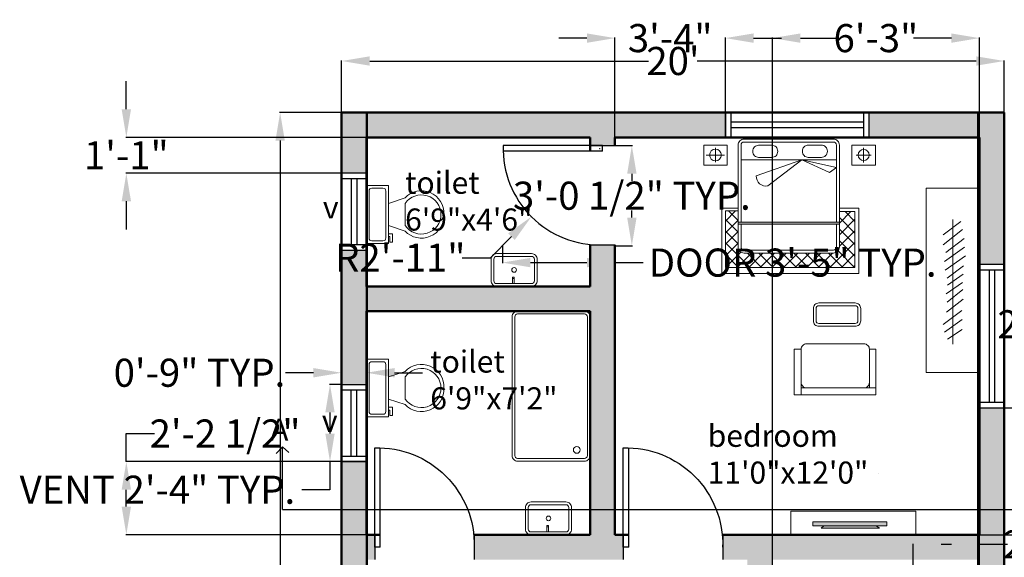
# Model space of a CAD drawing. Units: inches. Extents: x 4451 to 5261, y 886 to 1442.
# Tile 2 of 4: x 4451 to 4807, y 1247 to 1442. Entities that reach past the tile are written whole.
import ezdxf

# ---------------------------------------------------------------- set-up
doc = ezdxf.new("R2010")
doc.units = ezdxf.units.IN
doc.header["$MEASUREMENT"] = 0
for name, color, linetype, lineweight in [('A-ANNO-DIMS', 2, 'Continuous', 18), ('A-ANNO-SYMB', 3, 'Continuous', 25), ('A-ANNO-TEXT', 7, 'Continuous', 25), ('A-AREA-IDEN', 7, 'Continuous', 25), ('A-DOOR', 4, 'Continuous', 25), ('A-FLOR-FIXT', 9, 'Continuous', 20), ('A-FURN', 8, 'Continuous', 18), ('A-FURN-PATT', 8, 'Continuous', 13), ('A-GLAZ', 4, 'Continuous', 25), ('A-WALL', 7, 'Continuous', 50), ('A-WALL-PATT', 252, 'Continuous', 13)]:
    doc.layers.add(name, color=color, linetype=linetype, lineweight=lineweight)
doc.styles.get("Standard").update_dxf_attribs({"font": 'arial.ttf'})
doc.dimstyles.get("Standard").update_dxf_attribs({"dimtxt": 10.18, "dimasz": 10.18, "dimexe": 0.18, "dimexo": 0.0625, "dimgap": 0.09, "dimtad": 0, "dimtih": 1, "dimtoh": 1, "dimdec": 0, "dimzin": 0, "dimdsep": 46, "dimlunit": 3, "dimtxsty": 'Standard', "dimcen": 0.09, "dimadec": 0, "dimazin": 0, "dimtfac": 1, "dimtdec": 0, "dimtofl": 0, "dimtmove": 0, "dimatfit": 3, "dimfxl": 1, "dimtolj": 1, "dimtzin": 0, "dimarcsym": 0})
pattern_1 = [(45, (-374.59908, -99.02593), (-0.095474584, 0.095474584), []), (135, (-374.59908, -99.02593), (-0.2864237525, 0.095474584), [0.33755363, -0.202532178])]

# ---------------------------------------------------------------- blocks, each defined once
blk = doc.blocks.new('*U3')
for p, q in [((9.5, -6), (9.5, -2)), ((-10, -8.5), (-8, -8.5)), ((-10, -9.5), (-10, -8.5)), ((-7, -9.5), (-10, -9.5)), ((-8, -8.5), (-8, -8)), ((-7, -8), (-7, -9.5)), ((-4, -8), (-6, -14)), ((4, -8), (6, -14)), ((4, -14), (-4, -14))]:
    blk.add_line(p, q)
blk.add_lwpolyline([(10.5, -8), (10.5, 0), (-10.5, 0), (-10.5, -8)], close=True)
for points in [[(-9.5, -2), (-9.5, -6)], [(8.5, -1), (-8.5, -1)], [(-8.5, -7), (8.5, -7)]]:
    blk.add_lwpolyline(points)
for centre, radius, start, end in [((-8.625, -1.875), 0.8839, 81.8699, 188.1301), ((8.625, -1.875), 0.8839, 351.8699, 98.1301), ((-8.625, -6.125), 0.8839, 171.869898, 278.1301), ((8.625, -6.125), 0.8839, 261.8699, 8.1301), ((-0.4772, -19.9188), 8.0953, 133.01722, 273.38), ((0.0374, -19.8731), 7.127, 124.50543, 269.7), ((-0.0373, -19.8731), 7.127, 270.3, 55.4946), ((0.4773, -19.9188), 8.0953, 266.62, 46.9828)]:
    blk.add_arc(centre, radius, start, end)
blk = doc.blocks.new('*D11')
at = {"layer": 'A-ANNO-DIMS', "color": 0, "lineweight": -2, "transparency": 16777216}
for p, q in [((4567.09, 1408.31), (4567.09, 1427.09)), ((4577.27, 1426.91), (4678.28, 1426.91)), ((4796.91, 1426.91), (4695.91, 1426.91)), ((4807.09, 1408.31), (4807.09, 1427.09))]:
    blk.add_line(p, q, dxfattribs=at)
at = {"layer": 'A-ANNO-DIMS', "color": 0, "transparency": 16777216}
for points in [[(4577.27, 1428.6), (4577.27, 1425.21), (4567.09, 1426.91)], [(4796.91, 1428.6), (4796.91, 1425.21), (4807.09, 1426.91)]]:
    blk.add_solid(points, dxfattribs=at)
at = {"layer": 'Defpoints', "color": 0, "transparency": 16777216}
for p in [(4807.09, 1426.91), (4567.09, 1408.25), (4807.09, 1408.25)]:
    blk.add_point(p, dxfattribs=at)
at = {"layer": 'A-ANNO-DIMS', "color": 0, "transparency": 16777216, "insert": (4687.09, 1426.91), "char_height": 10.18, "attachment_point": 5}
blk.add_mtext("\\A1;20'", dxfattribs=at)
blk = doc.blocks.new('*D12')
at = {"layer": 'A-ANNO-DIMS', "color": 0, "lineweight": -2, "transparency": 16777216}
for p, q in [((4567.03, 1408.25), (4544.66, 1408.25)), ((4544.84, 1398.07), (4544.84, 1173.54)), ((4544.84, 938.43), (4544.84, 1162.96)), ((4567.03, 928.25), (4544.66, 928.25))]:
    blk.add_line(p, q, dxfattribs=at)
at = {"layer": 'A-ANNO-DIMS', "color": 0, "transparency": 16777216}
for points in [[(4543.14, 1398.07), (4546.53, 1398.07), (4544.84, 1408.25)], [(4543.14, 938.43), (4546.53, 938.43), (4544.84, 928.25)]]:
    blk.add_solid(points, dxfattribs=at)
at = {"layer": 'Defpoints', "color": 0, "transparency": 16777216}
for p in [(4567.09, 1408.25), (4544.84, 928.25), (4567.09, 928.25)]:
    blk.add_point(p, dxfattribs=at)
at = {"layer": 'A-ANNO-DIMS', "color": 0, "transparency": 16777216, "insert": (4544.84, 1168.25), "char_height": 10.18, "attachment_point": 5}
blk.add_mtext("\\A1;40'", dxfattribs=at)
blk = doc.blocks.new('DOOR-36-SWING')
for p, q in [((36.01, 36.01), (0.01, 36.01)), ((31.51, 36.01), (40.51, 36.01)), ((36.01, 34.01), (36.01, 36.01)), ((36.01, 34.01), (0.01, 34.01)), ((31.51, 0.01), (40.51, 0.01))]:
    blk.add_line(p, q)
blk.add_arc((35.01, 35.01), 35.01, 178.3634, 271.6366)
blk = doc.blocks.new('WIN-48-PLAN')
for p, q in [((0, 52), (9, 52)), ((0, 50), (9, 50)), ((3.5, 50), (3.5, 2)), ((5.5, 50), (5.5, 2)), ((0, 2), (9, 2)), ((0, 0), (9, 0))]:
    blk.add_line(p, q)
blk = doc.blocks.new('VENT-24-PLAN')
for p, q in [((9, 28), (0, 28)), ((9, 26), (0, 26)), ((3.5, 26), (3.5, 2)), ((5.5, 26), (5.5, 2)), ((9, 2), (0, 2)), ((9, 0), (0, 0))]:
    blk.add_line(p, q)
blk = doc.blocks.new('*D23')
at = {"layer": 'A-ANNO-DIMS', "color": 0, "lineweight": -2, "transparency": 16777216}
for p, q in [((4625.32, 1359.91), (4625.32, 1353.68)), ((4666.09, 1359.91), (4666.09, 1353.68)), ((4635.5, 1353.86), (4655.91, 1353.86)), ((4666.09, 1353.86), (4676.27, 1353.86))]:
    blk.add_line(p, q, dxfattribs=at)
at = {"layer": 'A-ANNO-DIMS', "color": 0, "transparency": 16777216}
for points in [[(4635.5, 1355.56), (4635.5, 1352.16), (4625.32, 1353.86)], [(4655.91, 1355.56), (4655.91, 1352.16), (4666.09, 1353.86)]]:
    blk.add_solid(points, dxfattribs=at)
at = {"layer": 'Defpoints', "color": 0, "transparency": 16777216}
for p in [(4625.32, 1359.98), (4666.09, 1359.98), (4666.09, 1353.86)]:
    blk.add_point(p, dxfattribs=at)
at = {"layer": 'A-ANNO-DIMS', "color": 0, "transparency": 16777216, "insert": (4730.44, 1353.86), "char_height": 10.18, "attachment_point": 5}
blk.add_mtext('\\A1;DOOR 3\'-5" TYP.', dxfattribs=at)
blk = doc.blocks.new('*D24')
at = {"layer": 'A-ANNO-DIMS', "color": 0, "lineweight": -2, "transparency": 16777216}
for p, q in [((4666.16, 1396.25), (4672.39, 1396.25)), ((4672.21, 1386.07), (4672.21, 1383.47)), ((4672.21, 1370.16), (4672.21, 1372.76)), ((4666.16, 1359.98), (4672.39, 1359.98))]:
    blk.add_line(p, q, dxfattribs=at)
at = {"layer": 'A-ANNO-DIMS', "color": 0, "transparency": 16777216}
for points in [[(4670.51, 1386.07), (4673.91, 1386.07), (4672.21, 1396.25)], [(4670.51, 1370.16), (4673.91, 1370.16), (4672.21, 1359.98)]]:
    blk.add_solid(points, dxfattribs=at)
at = {"layer": 'Defpoints', "color": 0, "transparency": 16777216}
for p in [(4666.09, 1396.25), (4672.21, 1396.25), (4666.09, 1359.98)]:
    blk.add_point(p, dxfattribs=at)
at = {"layer": 'A-ANNO-DIMS', "color": 0, "transparency": 16777216, "insert": (4672.21, 1378.11), "char_height": 10.18, "attachment_point": 5}
blk.add_mtext('\\A1;3\'-0 1/2" TYP.', dxfattribs=at)
blk = doc.blocks.new('*D25')
at = {"layer": 'A-ANNO-DIMS', "color": 0, "lineweight": -2, "transparency": 16777216}
for p, q in [((4567.03, 1309.75), (4562.71, 1309.75)), ((4562.89, 1299.57), (4562.89, 1291.93)), ((4567.03, 1281.75), (4562.71, 1281.75)), ((4562.89, 1281.75), (4562.89, 1271.57)), ((4562.89, 1271.57), (4552.71, 1271.57))]:
    blk.add_line(p, q, dxfattribs=at)
at = {"layer": 'A-ANNO-DIMS', "color": 0, "transparency": 16777216}
for points in [[(4561.2, 1299.57), (4564.59, 1299.57), (4562.89, 1309.75)], [(4561.2, 1291.93), (4564.59, 1291.93), (4562.89, 1281.75)]]:
    blk.add_solid(points, dxfattribs=at)
at = {"layer": 'Defpoints', "color": 0, "transparency": 16777216}
for p in [(4567.09, 1309.75), (4562.89, 1281.75), (4567.09, 1281.75)]:
    blk.add_point(p, dxfattribs=at)
at = {"layer": 'A-ANNO-DIMS', "color": 0, "transparency": 16777216, "insert": (4500.39, 1271.57), "char_height": 10.18, "attachment_point": 5}
blk.add_mtext('\\A1;VENT 2\'-4" TYP.', dxfattribs=at)
blk = doc.blocks.new('*D26')
at = {"layer": 'A-ANNO-DIMS', "color": 0, "lineweight": -2, "transparency": 16777216}
for p, q in [((4556.91, 1313.95), (4546.73, 1313.95)), ((4567.09, 1309.81), (4567.09, 1314.13)), ((4576.09, 1309.81), (4576.09, 1314.13)), ((4586.27, 1313.95), (4596.45, 1313.95))]:
    blk.add_line(p, q, dxfattribs=at)
at = {"layer": 'A-ANNO-DIMS', "color": 0, "transparency": 16777216}
for points in [[(4556.91, 1315.65), (4556.91, 1312.26), (4567.09, 1313.95)], [(4586.27, 1315.65), (4586.27, 1312.26), (4576.09, 1313.95)]]:
    blk.add_solid(points, dxfattribs=at)
at = {"layer": 'Defpoints', "color": 0, "transparency": 16777216}
for p in [(4567.09, 1313.95), (4567.09, 1309.75), (4576.09, 1309.75)]:
    blk.add_point(p, dxfattribs=at)
at = {"layer": 'A-ANNO-DIMS', "color": 0, "transparency": 16777216, "insert": (4515.62, 1313.95), "char_height": 10.18, "attachment_point": 5}
blk.add_mtext('\\A1;0\'-9" TYP.', dxfattribs=at)
blk = doc.blocks.new('*D41')
at = {"layer": 'A-ANNO-DIMS', "color": 0, "lineweight": -2, "transparency": 16777216}
for p, q in [((4723.09, 1102.31), (4723.09, 1435.38)), ((4733.27, 1435.2), (4746.94, 1435.2)), ((4787.91, 1435.2), (4774.24, 1435.2)), ((4798.09, 1102.31), (4798.09, 1435.38))]:
    blk.add_line(p, q, dxfattribs=at)
at = {"layer": 'A-ANNO-DIMS', "color": 0, "transparency": 16777216}
for points in [[(4733.27, 1436.9), (4733.27, 1433.51), (4723.09, 1435.2)], [(4787.91, 1436.9), (4787.91, 1433.51), (4798.09, 1435.2)]]:
    blk.add_solid(points, dxfattribs=at)
at = {"layer": 'Defpoints', "color": 0, "transparency": 16777216}
for p in [(4798.09, 1435.2), (4723.09, 1102.25), (4798.09, 1102.25)]:
    blk.add_point(p, dxfattribs=at)
at = {"layer": 'A-ANNO-DIMS', "color": 0, "transparency": 16777216, "insert": (4760.59, 1435.2), "char_height": 10.18, "attachment_point": 5}
blk.add_mtext('\\A1;6\'-3"', dxfattribs=at)
blk = doc.blocks.new('*D46')
at = {"layer": 'A-ANNO-DIMS', "color": 0, "lineweight": -2, "transparency": 16777216}
for p, q in [((4798.16, 1301.25), (4859.61, 1301.25)), ((4859.43, 1291.07), (4859.43, 1283.54)), ((4859.43, 1265.43), (4859.43, 1272.96)), ((4798.16, 1255.25), (4859.61, 1255.25))]:
    blk.add_line(p, q, dxfattribs=at)
at = {"layer": 'A-ANNO-DIMS', "color": 0, "transparency": 16777216}
for points in [[(4857.74, 1291.07), (4861.13, 1291.07), (4859.43, 1301.25)], [(4857.74, 1265.43), (4861.13, 1265.43), (4859.43, 1255.25)]]:
    blk.add_solid(points, dxfattribs=at)
at = {"layer": 'Defpoints', "color": 0, "transparency": 16777216}
for p in [(4798.09, 1301.25), (4859.43, 1301.25), (4798.09, 1255.25)]:
    blk.add_point(p, dxfattribs=at)
at = {"layer": 'A-ANNO-DIMS', "color": 0, "transparency": 16777216, "insert": (4859.43, 1278.25), "char_height": 10.18, "attachment_point": 5}
blk.add_mtext('\\A1;3\'-10"', dxfattribs=at)
blk = doc.blocks.new('*D47')
at = {"layer": 'A-ANNO-DIMS', "color": 0, "lineweight": -2, "transparency": 16777216}
for p, q in [((4655.91, 1435.2), (4645.73, 1435.2)), ((4666.09, 1399.31), (4666.09, 1435.38)), ((4706.09, 1399.31), (4706.09, 1435.38)), ((4716.27, 1435.2), (4726.45, 1435.2))]:
    blk.add_line(p, q, dxfattribs=at)
at = {"layer": 'A-ANNO-DIMS', "color": 0, "transparency": 16777216}
for points in [[(4655.91, 1436.9), (4655.91, 1433.51), (4666.09, 1435.2)], [(4716.27, 1436.9), (4716.27, 1433.51), (4706.09, 1435.2)]]:
    blk.add_solid(points, dxfattribs=at)
at = {"layer": 'Defpoints', "color": 0, "transparency": 16777216}
for p in [(4706.09, 1435.2), (4666.09, 1399.25), (4706.09, 1399.25)]:
    blk.add_point(p, dxfattribs=at)
at = {"layer": 'A-ANNO-DIMS', "color": 0, "transparency": 16777216, "insert": (4686.09, 1435.2), "char_height": 10.18, "attachment_point": 5}
blk.add_mtext('\\A1;3\'-4"', dxfattribs=at)
blk = doc.blocks.new('*D49')
at = {"layer": 'A-ANNO-DIMS', "color": 0, "lineweight": -2, "transparency": 16777216}
for p, q in [((4489.14, 1281.75), (4489.14, 1291.93)), ((4489.14, 1291.93), (4499.32, 1291.93)), ((4576.03, 1281.75), (4488.96, 1281.75)), ((4489.14, 1265.43), (4489.14, 1271.57)), ((4576.03, 1255.25), (4488.96, 1255.25))]:
    blk.add_line(p, q, dxfattribs=at)
at = {"layer": 'A-ANNO-DIMS', "color": 0, "transparency": 16777216}
for points in [[(4487.45, 1271.57), (4490.84, 1271.57), (4489.14, 1281.75)], [(4487.45, 1265.43), (4490.84, 1265.43), (4489.14, 1255.25)]]:
    blk.add_solid(points, dxfattribs=at)
at = {"layer": 'Defpoints', "color": 0, "transparency": 16777216}
for p in [(4489.14, 1281.75), (4576.09, 1281.75), (4576.09, 1255.25)]:
    blk.add_point(p, dxfattribs=at)
at = {"layer": 'A-ANNO-DIMS', "color": 0, "transparency": 16777216, "insert": (4524.89, 1291.93), "char_height": 10.18, "attachment_point": 5}
blk.add_mtext('\\A1;2\'-2 1/2"', dxfattribs=at)
blk = doc.blocks.new('*D50')
at = {"layer": 'A-ANNO-DIMS', "color": 0, "lineweight": -2, "transparency": 16777216}
for p, q in [((4489.14, 1409.43), (4489.14, 1419.61)), ((4576.03, 1399.25), (4488.96, 1399.25)), ((4576.03, 1386.25), (4488.96, 1386.25)), ((4489.14, 1376.07), (4489.14, 1365.89))]:
    blk.add_line(p, q, dxfattribs=at)
at = {"layer": 'A-ANNO-DIMS', "color": 0, "transparency": 16777216}
for points in [[(4487.45, 1409.43), (4490.84, 1409.43), (4489.14, 1399.25)], [(4487.45, 1376.07), (4490.84, 1376.07), (4489.14, 1386.25)]]:
    blk.add_solid(points, dxfattribs=at)
at = {"layer": 'Defpoints', "color": 0, "transparency": 16777216}
for p in [(4576.09, 1399.25), (4489.14, 1386.25), (4576.09, 1386.25)]:
    blk.add_point(p, dxfattribs=at)
at = {"layer": 'A-ANNO-DIMS', "color": 0, "transparency": 16777216, "insert": (4489.14, 1392.75), "char_height": 10.18, "attachment_point": 5}
blk.add_mtext('\\A1;1\'-1"', dxfattribs=at)
blk = doc.blocks.new('*D54')
at = {"layer": 'A-ANNO-DIMS', "color": 0, "lineweight": -2, "transparency": 16777216}
for p, q in [((4774.09, 1224.89), (4774.09, 1251.96)), ((4784.27, 1251.78), (4787.91, 1251.78)), ((4798.09, 1224.89), (4798.09, 1251.96)), ((4798.09, 1251.78), (4808.27, 1251.78))]:
    blk.add_line(p, q, dxfattribs=at)
at = {"layer": 'A-ANNO-DIMS', "color": 0, "transparency": 16777216}
for points in [[(4784.27, 1253.48), (4784.27, 1250.08), (4774.09, 1251.78)], [(4787.91, 1253.48), (4787.91, 1250.08), (4798.09, 1251.78)]]:
    blk.add_solid(points, dxfattribs=at)
at = {"layer": 'Defpoints', "color": 0, "transparency": 16777216}
for p in [(4798.09, 1251.78), (4774.09, 1224.83), (4798.09, 1224.83)]:
    blk.add_point(p, dxfattribs=at)
at = {"layer": 'A-ANNO-DIMS', "color": 0, "transparency": 16777216, "insert": (4821.98, 1251.78), "char_height": 10.18, "attachment_point": 5}
blk.add_mtext('\\A1;2\'-0"', dxfattribs=at)
blk = doc.blocks.new('*D61')
at = {"layer": 'A-ANNO-DIMS', "color": 0, "lineweight": -2, "transparency": 16777216}
for p, q in [((4860.41, 1349.3), (4835.61, 1349.3)), ((4835.79, 1339.12), (4835.79, 1336.87)), ((4835.79, 1323.9), (4835.79, 1326.16)), ((4880.22, 1313.72), (4835.61, 1313.72))]:
    blk.add_line(p, q, dxfattribs=at)
at = {"layer": 'A-ANNO-DIMS', "color": 0, "transparency": 16777216}
for points in [[(4834.09, 1339.12), (4837.48, 1339.12), (4835.79, 1349.3)], [(4834.09, 1323.9), (4837.48, 1323.9), (4835.79, 1313.72)]]:
    blk.add_solid(points, dxfattribs=at)
at = {"layer": 'Defpoints', "color": 0, "transparency": 16777216}
for p in [(4835.79, 1349.3), (4860.47, 1349.3), (4880.28, 1313.72)]:
    blk.add_point(p, dxfattribs=at)
at = {"layer": 'A-ANNO-DIMS', "color": 0, "transparency": 16777216, "insert": (4835.79, 1331.51), "char_height": 10.18, "attachment_point": 5}
blk.add_mtext('\\A1;2\'-11 1/2"', dxfattribs=at)
blk = doc.blocks.new('*D81')
at = {"layer": 'A-ANNO-DIMS', "color": 0, "lineweight": -2, "transparency": 16777216}
for p, q in [((4660.5, 1395.25), (4660.68, 1395.25)), ((4660.59, 1395.16), (4660.59, 1395.34)), ((4620.98, 1355.64), (4628.64, 1363.3)), ((4610.8, 1355.64), (4620.98, 1355.64))]:
    blk.add_line(p, q, dxfattribs=at)
at = {"layer": 'A-ANNO-DIMS', "color": 0, "transparency": 16777216}
blk.add_solid([(4627.44, 1364.49), (4629.84, 1362.1), (4635.83, 1370.49)], dxfattribs=at)
at = {"layer": 'Defpoints', "color": 0, "transparency": 16777216}
for p in [(4660.59, 1395.25), (4635.83, 1370.49)]:
    blk.add_point(p, dxfattribs=at)
at = {"layer": 'A-ANNO-DIMS', "color": 0, "transparency": 16777216, "insert": (4588.35, 1355.64), "char_height": 10.18, "attachment_point": 5}
blk.add_mtext('\\A1;R2\'-11"', dxfattribs=at)

msp = doc.modelspace()

# ---------------------------------------------------------------- hatches: boundary and pattern name
at = {"layer": 'A-FURN-PATT'}
h = msp.add_hatch(dxfattribs=at)
h.set_pattern_fill('ANSI37', color=256, scale=23.763776)
h.set_pattern_definition([(45, (-374.599, -99.026), (-2.1004409, 2.1004409), []), (135, (-374.599, -99.026), (-2.1004409, -2.1004409), [])])
h.paths.add_polyline_path([(4753, 1352.14), (4753, 1372.36), (4747.37, 1372.36), (4747.37, 1359.46, -0.414214), (4745.2, 1357.3), (4712.84, 1357.3, -0.414214), (4710.68, 1359.46), (4710.68, 1372.58), (4706.09, 1372.58), (4706.09, 1352.14)])
h = msp.add_hatch(dxfattribs=at)
h.set_pattern_fill('ANSI38', color=256, scale=1.080172)
h.set_pattern_definition(pattern_1)
h.paths.add_polyline_path([(4711.76, 1368.56), (4710.68, 1368.56), (4710.68, 1367.77), (4711.76, 1367.77)])
h.paths.add_polyline_path([(4747.37, 1368.56), (4746.29, 1368.56), (4746.29, 1367.77), (4747.37, 1367.77)])
h = msp.add_hatch(dxfattribs=at)
h.set_pattern_fill('ANSI38', color=256, scale=1.080172)
h.set_pattern_definition(pattern_1)
h.paths.add_polyline_path([(4746.29, 1368.56), (4711.76, 1368.56), (4711.76, 1367.77), (4746.29, 1367.77)])
h = msp.add_hatch(color=256, dxfattribs=at)
h.dxf.hatch_style = 1
h.paths.add_polyline_path([(4764.53, 1259.92), (4737.8, 1259.92), (4737.8, 1258.54), (4764.53, 1258.54)])
h.paths.add_polyline_path([(4760.66, 1258.54), (4741.71, 1258.54), (4740.83, 1257.67), (4761.95, 1257.67)])
at = {"layer": 'A-WALL-PATT'}
h = msp.add_hatch(color=256, dxfattribs=at)
h.dxf.hatch_style = 1
h.paths.add_polyline_path([(4706.09, 1408.25), (4567.09, 1408.25), (4567.09, 1386.25), (4576.09, 1386.25), (4576.09, 1399.25), (4657.09, 1399.25), (4657.09, 1396.25), (4661.59, 1396.25), (4666.09, 1396.25), (4666.09, 1399.25), (4706.09, 1399.25)])
h.paths.add_polyline_path([(4807.09, 1408.25), (4758.09, 1408.25), (4758.09, 1399.25), (4798.09, 1399.25), (4798.09, 1353.25), (4807.09, 1353.25)])
h.paths.add_polyline_path([(4807.09, 1301.25), (4798.09, 1301.25), (4798.09, 1292.89), (4798.09, 1255.25), (4705.09, 1255.25), (4705.09, 1252.75, -0.014283), (4705.09, 1250.75), (4705.09, 1246.25), (4714.09, 1246.25), (4714.09, 1243.25), (4723.09, 1243.25), (4723.09, 1246.25), (4798.09, 1246.25), (4798.09, 1200.25), (4807.09, 1200.25)])
h.paths.add_polyline_path([(4666.09, 1360.25), (4661.59, 1360.25, -0.014283), (4659.59, 1360.25), (4657.09, 1360.25), (4657.09, 1345.25), (4576.09, 1345.25), (4576.09, 1358.25), (4567.09, 1358.25), (4567.09, 1309.75), (4576.09, 1309.75), (4576.09, 1336.25), (4657.09, 1336.25), (4657.09, 1255.25), (4615.09, 1255.25), (4615.09, 1252.75, -0.014283), (4615.09, 1250.75), (4615.09, 1246.25), (4669.09, 1246.25), (4669.09, 1255.25), (4666.09, 1255.25)])
h.paths.add_polyline_path([(4576.09, 1281.75), (4567.09, 1281.75), (4567.09, 1211.26), (4576.09, 1211.26), (4576.09, 1246.25), (4579.09, 1246.25), (4579.09, 1255.25), (4576.09, 1255.25)])
h.paths.add_polyline_path([(4666.09, 1102.25), (4576.09, 1102.25), (4576.09, 1159.26), (4567.09, 1159.26), (4567.09, 928.25), (4596.54, 928.25), (4596.54, 937.25), (4576.09, 937.25), (4576.09, 1093.25), (4579.09, 1093.25), (4657.09, 1093.25), (4657.09, 982.46), (4666.09, 982.46), (4666.09, 1093.25)])
h.paths.add_polyline_path([(4723.09, 1207.25), (4720.59, 1207.25, -0.014283), (4718.59, 1207.25), (4714.09, 1207.25), (4714.09, 1102.25), (4711.09, 1102.25), (4711.09, 1097.75), (4711.09, 1093.25), (4734.59, 1093.25), (4734.59, 1102.25), (4723.09, 1102.25)])
h.paths.add_polyline_path([(4807.09, 1148.25), (4798.09, 1148.25), (4798.09, 1102.25), (4786.59, 1102.25), (4786.59, 1093.25), (4798.09, 1093.25), (4798.09, 1041.25), (4807.09, 1041.25)])
h.paths.add_polyline_path([(4694.85, 937.25), (4649.53, 937.25), (4648.54, 937.25), (4648.54, 928.25), (4649.53, 928.25), (4694.85, 928.25)])
h.paths.add_polyline_path([(4807.09, 989.25), (4798.09, 989.25), (4798.09, 937.25), (4798.09, 928.25), (4807.09, 928.25)])
h.paths.add_polyline_path([(4662.88, 1033.63), (4722.94, 1033.63), (4722.94, 1063.48), (4662.88, 1063.48)], flags=9)

# ---------------------------------------------------------------- linework, layer by layer
at = {"layer": 'A-ANNO-SYMB'}
for p, q in [((4545.71, 1287.14), (4543.39, 1284.64)), ((4545.71, 1264.36), (4545.71, 1287.14)), ((4545.71, 1287.14), (4547.97, 1285.05)), ((4545.71, 1264.36), (4671.09, 1264.36)), ((4671.09, 1264.36), (4828.9, 1264.36))]:
    msp.add_line(p, q, dxfattribs=at)
at = {"layer": 'A-FLOR-FIXT'}
for points in [[(4621.23, 1355.12, -0.414214), (4623.23, 1357.12), (4635.9, 1357.12, -0.414214), (4637.9, 1355.12), (4637.9, 1347.25, -0.414214), (4635.9, 1345.25), (4623.23, 1345.25, -0.414214), (4621.23, 1347.25)], [(4622.23, 1355.12, -0.414214), (4623.23, 1356.12), (4635.9, 1356.12, -0.414214), (4636.9, 1355.12), (4636.9, 1347.25, -0.414214), (4635.9, 1346.25), (4623.23, 1346.25, -0.414214), (4622.23, 1347.25)], [(4657.09, 1334.25, 0.414214), (4655.09, 1336.25), (4630.84, 1336.25, 0.414214), (4628.84, 1334.25), (4628.84, 1283.91, 0.414214), (4630.84, 1281.91), (4655.09, 1281.91, 0.414214), (4657.09, 1283.91)], [(4656.09, 1334.25, 0.414214), (4655.09, 1335.25), (4630.84, 1335.25, 0.414214), (4629.84, 1334.25), (4629.84, 1283.91, 0.414214), (4630.84, 1282.91), (4655.09, 1282.91, 0.414214), (4656.09, 1283.91)], [(4633.69, 1265.12, -0.414214), (4635.69, 1267.12), (4648.35, 1267.12, -0.414214), (4650.35, 1265.12), (4650.35, 1257.25, -0.414214), (4648.35, 1255.25), (4635.69, 1255.25, -0.414214), (4633.69, 1257.25)], [(4634.69, 1265.12, -0.414214), (4635.69, 1266.12), (4648.35, 1266.12, -0.414214), (4649.35, 1265.12), (4649.35, 1257.25, -0.414214), (4648.35, 1256.25), (4635.69, 1256.25, -0.414214), (4634.69, 1257.25)]]:
    msp.add_lwpolyline(points, format="xyb", close=True, dxfattribs=at)
for points in [[(4629.57, 1346.25), (4629.57, 1346.25), (4629.01, 1346.25), (4629.01, 1346.25), (4629.01, 1348.57), (4629.01, 1348.57), (4629.57, 1348.57), (4629.57, 1348.57)], [(4629.01, 1348.57), (4629.01, 1348.57), (4629.57, 1348.57), (4629.57, 1348.57), (4629.57, 1348.09), (4629.57, 1348.09), (4629.01, 1348.09), (4629.01, 1348.09)], [(4642.02, 1256.25), (4642.02, 1256.25), (4641.46, 1256.25), (4641.46, 1256.25), (4641.46, 1258.57), (4641.46, 1258.57), (4642.02, 1258.57), (4642.02, 1258.57)], [(4641.46, 1258.57), (4641.46, 1258.57), (4642.02, 1258.57), (4642.02, 1258.57), (4642.02, 1258.09), (4642.02, 1258.09), (4641.46, 1258.09), (4641.46, 1258.09)]]:
    msp.add_lwpolyline(points, close=True, dxfattribs=at)
for centre, radius in [((4629.57, 1351.19), 0.842), ((4652.26, 1286), 1.24), ((4642.02, 1261.19), 0.842)]:
    msp.add_circle(centre, radius, dxfattribs=at)
at = {"layer": 'A-FURN'}
for p, q in [((4702.49, 1395.43), (4702.49, 1390.2)), ((4756.16, 1395.39), (4756.16, 1390.13)), ((4699.09, 1392.84), (4705.75, 1392.84)), ((4733.74, 1391.08), (4717.27, 1385.27)), ((4721.43, 1381.68), (4733.74, 1391.08)), ((4746.29, 1388.3), (4733.74, 1391.08)), ((4733.74, 1391.08), (4743.74, 1386.47)), ((4753.49, 1392.76), (4758.93, 1392.76)), ((4743.74, 1386.47), (4746.29, 1388.3)), ((4710.68, 1373.61), (4704.82, 1373.61)), ((4704.82, 1373.61), (4704.82, 1349.9)), ((4710.68, 1373.61), (4710.68, 1373.61)), ((4754.45, 1373.61), (4747.37, 1373.61)), ((4754.45, 1349.9), (4754.45, 1373.61)), ((4710.68, 1372.58), (4706.09, 1372.58)), ((4706.09, 1372.58), (4706.09, 1352.14)), ((4747.37, 1372.36), (4753, 1372.36)), ((4753, 1372.36), (4753, 1352.14)), ((4788.46, 1369.51), (4788.46, 1324.32)), ((4710.68, 1368.56), (4747.37, 1368.56)), ((4710.68, 1367.77), (4747.37, 1367.77)), ((4785.01, 1363.88), (4791.36, 1368.8)), ((4785.01, 1360.32), (4791.9, 1365.88)), ((4785.9, 1357.5), (4792.6, 1362.65)), ((4785.44, 1354.28), (4792.67, 1359.5)), ((4785.67, 1351.13), (4793.06, 1356.27)), ((4706.09, 1352.14), (4753, 1352.14)), ((4786.44, 1348.28), (4792.36, 1352.66)), ((4704.82, 1349.9), (4754.45, 1349.9)), ((4786.55, 1345.65), (4792.21, 1349.66)), ((4785.99, 1342.51), (4791.96, 1346.62)), ((4786.43, 1339.53), (4792.11, 1344.12)), ((4786.14, 1335.91), (4792.16, 1340.6)), ((4784.95, 1331.43), (4791.71, 1336.55)), ((4785.48, 1328.62), (4791.87, 1333.26)), ((4786.47, 1326.14), (4791.82, 1329.65)), ((4760.51, 1308.43), (4760.51, 1305.99)), ((4741.71, 1258.54), (4739.83, 1258.54)), ((4741.71, 1258.54), (4740.83, 1257.67)), ((4740.83, 1257.67), (4761.95, 1257.67)), ((4761.95, 1257.67), (4760.66, 1258.54))]:
    msp.add_line(p, q, dxfattribs=at)
for points in [[(4710.68, 1396.46, -0.414214), (4712.84, 1398.62), (4745.2, 1398.62, -0.414214), (4747.37, 1396.46), (4747.37, 1359.46, -0.414214), (4745.2, 1357.3), (4712.84, 1357.3, -0.414214), (4710.68, 1359.46)], [(4715.97, 1394.23, -0.414214), (4718.13, 1396.39), (4722.89, 1396.39, -0.414214), (4725.05, 1394.23), (4725.05, 1394.13, -0.414214), (4722.89, 1391.97), (4718.13, 1391.97, -0.414214), (4715.97, 1394.13)], [(4733.95, 1394.24, -0.414214), (4736.11, 1396.41), (4740.87, 1396.41, -0.414214), (4743.03, 1394.24), (4743.03, 1394.15, -0.414214), (4740.87, 1391.99), (4736.11, 1391.99, -0.414214), (4733.95, 1394.15)], [(4737.94, 1337.25, -0.414214), (4739.94, 1339.25), (4753.08, 1339.25, -0.414214), (4755.08, 1337.25), (4755.08, 1332.78, -0.414214), (4753.08, 1330.78), (4739.94, 1330.78, -0.414214), (4737.94, 1332.78)], [(4738.94, 1337.25, -0.414214), (4739.94, 1338.25), (4753.08, 1338.25, -0.414214), (4754.08, 1337.25), (4754.08, 1332.78, -0.414214), (4753.08, 1331.78), (4739.94, 1331.78, -0.414214), (4738.94, 1332.78)], [(4733.54, 1322.44, -0.414214), (4735.54, 1324.44), (4756.25, 1324.44, -0.414214), (4758.25, 1322.44), (4758.25, 1310.45, -0.414214), (4756.25, 1308.45), (4735.54, 1308.45, -0.414214), (4733.54, 1310.45)]]:
    msp.add_lwpolyline(points, format="xyb", close=True, dxfattribs=at)
for points in [[(4698.22, 1396.46), (4698.22, 1396.46), (4706.75, 1396.46), (4706.75, 1396.46), (4706.75, 1389.21), (4706.75, 1389.21), (4698.22, 1389.21), (4698.22, 1389.21)], [(4751.9, 1396.46), (4751.9, 1396.46), (4760.42, 1396.46), (4760.42, 1396.46), (4760.42, 1389.21), (4760.42, 1389.21), (4751.9, 1389.21), (4751.9, 1389.21)], [(4711.76, 1391.08), (4711.76, 1391.08), (4746.29, 1391.08), (4746.29, 1391.08), (4746.29, 1391.08), (4746.29, 1391.08), (4711.76, 1391.08), (4711.76, 1391.08)], [(4798.09, 1380.8), (4798.09, 1380.8), (4778.83, 1380.8), (4778.83, 1380.8), (4778.83, 1314.01), (4778.83, 1314.01), (4798.09, 1314.01), (4798.09, 1314.01)], [(4733.54, 1322.44), (4733.54, 1322.44), (4730.95, 1322.44), (4730.95, 1322.44), (4730.95, 1305.99), (4730.95, 1305.99), (4733.54, 1305.99), (4733.54, 1305.99)], [(4758.25, 1322.44), (4758.25, 1322.44), (4760.51, 1322.44), (4760.51, 1322.44), (4760.51, 1308.43), (4760.51, 1308.43), (4758.25, 1308.43), (4758.25, 1308.43)], [(4761.38, 1277.4), (4761.38, 1277.4)], [(4775, 1255.25), (4775, 1255.25), (4729.77, 1255.25), (4729.77, 1255.25), (4729.77, 1263.8), (4729.77, 1263.8), (4775, 1263.8), (4775, 1263.8)], [(4737.8, 1259.92), (4737.8, 1259.92), (4764.53, 1259.92), (4764.53, 1259.92), (4764.53, 1258.54), (4764.53, 1258.54), (4737.8, 1258.54), (4737.8, 1258.54)]]:
    msp.add_lwpolyline(points, close=True, dxfattribs=at)
for points in [[(4711.76, 1368.56), (4711.76, 1396.46, -0.414214), (4712.84, 1397.54), (4745.2, 1397.54, -0.414214), (4746.29, 1396.46), (4746.29, 1368.56)], [(4746.29, 1367.77), (4746.29, 1359.46, -0.414214), (4745.2, 1358.38), (4712.84, 1358.38, -0.414214), (4711.76, 1359.46), (4711.76, 1367.77)]]:
    msp.add_lwpolyline(points, format="xyb", dxfattribs=at)
msp.add_lwpolyline([(4760.51, 1308.43), (4733.54, 1308.43), (4733.54, 1308.43), (4733.54, 1305.99), (4733.54, 1305.99), (4760.51, 1305.99)], dxfattribs=at)
for centre, radius in [((4702.49, 1392.84), 2.14), ((4756.16, 1392.84), 1.98)]:
    msp.add_circle(centre, radius, dxfattribs=at)
msp.add_arc((4720.76, 1385.1), 3.49, 177.2727, 281.0516, dxfattribs=at)
at = {"layer": 'A-WALL'}
for p, q in [((4567.09, 928.25), (4567.09, 1408.25)), ((4567.09, 1408.25), (4807.09, 1408.25)), ((4576.2, 928.25), (4576.2, 1408.25)), ((4797.65, 928.29), (4797.65, 1408.25)), ((4807.09, 1408.25), (4807.09, 928.25)), ((4576.09, 1399.25), (4657.09, 1399.25)), ((4576.09, 1345.25), (4576.09, 1399.25)), ((4657.09, 1394.25), (4657.09, 1399.25)), ((4666.09, 1399.25), (4798.09, 1399.25)), ((4666.09, 1396.25), (4666.09, 1399.25)), ((4798.09, 1399.25), (4798.09, 1255.25)), ((4798.09, 1380.8), (4798.09, 1292.89)), ((4657.09, 1345.25), (4657.09, 1360.41)), ((4666.09, 1255.25), (4666.09, 1360.25)), ((4576.09, 1345.25), (4657.09, 1345.25)), ((4576.09, 1336.25), (4657.09, 1336.25)), ((4576.09, 1255.25), (4576.09, 1336.25)), ((4657.09, 1255.25), (4657.09, 1336.25)), ((4576.09, 1255.25), (4581.09, 1255.25)), ((4614.93, 1255.25), (4657.09, 1255.25)), ((4666.09, 1255.25), (4671.09, 1255.25)), ((4704.93, 1255.25), (4798.09, 1255.25))]:
    msp.add_line(p, q, dxfattribs=at)

# ---------------------------------------------------------------- block references
at = {"layer": 'A-DOOR'}
msp.add_blockref('DOOR-36-SWING', (4625.58, 1360.24), dxfattribs=at)
at = {"layer": 'A-DOOR', "extrusion": (0, 0, -1), "zscale": -1}
for p, rotation in [((-4615.11, 1286.77), 269.9999999999958), ((-4705.11, 1286.77), 270.0000000000006)]:
    msp.add_blockref('DOOR-36-SWING', p, dxfattribs=dict(at, rotation=rotation))
at = {"layer": 'A-FLOR-FIXT', "rotation": 90}
for p in [(4576.09, 1371.3), (4576.09, 1308.43)]:
    msp.add_blockref('*U3', p, dxfattribs=at)
at = {"layer": 'A-GLAZ'}
for name, p, rotation in [('WIN-48-PLAN', (4706.09, 1408.25), 269.9999999999998), ('VENT-24-PLAN', (4576.09, 1309.75), 180)]:
    msp.add_blockref(name, p, dxfattribs=dict(at, rotation=rotation))
for name, p in [('VENT-24-PLAN', (4567.09, 1358.25)), ('WIN-48-PLAN', (4798.09, 1301.25))]:
    msp.add_blockref(name, p, dxfattribs=at)

# ---------------------------------------------------------------- texts
at = {"layer": 'A-ANNO-SYMB', "insert": (4541.22, 1297.32), "char_height": 8, "attachment_point": 1}
msp.add_mtext_dynamic_manual_height_columns('A', width=18.4117, gutter_width=1, heights=[0], dxfattribs=at)
at = {"layer": 'A-ANNO-TEXT', "char_height": 8, "attachment_point": 1}
for insert in [(4560.32, 1377.87), (4559.96, 1300.48)]:
    msp.add_mtext_dynamic_manual_height_columns('v', width=18.4117, gutter_width=1, heights=[0], dxfattribs=dict(at, insert=insert))
at = {"layer": 'A-AREA-IDEN', "char_height": 8, "attachment_point": 1}
for s, insert in [('toilet\\P6\'9"x4\'6"', (4590.09, 1386.8)), ('toilet\\P6\'9"x7\'2"', (4599.2, 1322.01)), ('bedroom\\P11\'0"x12\'0"', (4699.66, 1295.11))]:
    msp.add_mtext_dynamic_manual_height_columns(s, width=82.2612, gutter_width=1, heights=[0], dxfattribs=dict(at, insert=insert))

# ---------------------------------------------------------------- dimensions: what is measured, and where the dimension line sits
at = {"layer": 'A-ANNO-DIMS'}
for base, p1, p2, override, picture, middle in [((4706.09, 1435.2), (4666.09, 1399.25), (4706.09, 1399.25), {"dimdec": 1, "dimlfac": 1, "dimrnd": 0, "dimzin": 1, "dimdsep": 46, "dimlunit": 4, "dimfrac": 2}, '*D47', (4686.09, 1435.2)), ((4798.09, 1435.2), (4723.09, 1102.25), (4798.09, 1102.25), {"dimdec": 1, "dimlfac": 1, "dimrnd": 0, "dimzin": 1, "dimdsep": 46, "dimlunit": 4, "dimfrac": 2}, '*D41', (4760.59, 1435.2)), ((4807.09, 1426.91), (4567.09, 1408.25), (4807.09, 1408.25), {"dimclrd": 0, "dimclre": 0, "dimclrt": 0}, '*D11', (4687.09, 1426.91)), ((4798.09, 1251.78), (4774.09, 1224.83), (4798.09, 1224.83), {"dimdec": 1, "dimlfac": 1, "dimrnd": 0, "dimzin": 1, "dimdsep": 46, "dimlunit": 4, "dimfrac": 2}, '*D54', (4821.98, 1251.78))]:
    dim = msp.add_linear_dim(base=base, p1=p1, p2=p2, dimstyle='Standard', override=override, dxfattribs=at)
    dim.commit()
    dim.dimension.update_dxf_attribs({"geometry": picture, "text_midpoint": middle})
for base, p1, p2, override, picture, middle in [((4489.14, 1386.25), (4576.09, 1399.25), (4576.09, 1386.25), {"dimdec": 1, "dimlfac": 1, "dimrnd": 0, "dimzin": 1, "dimdsep": 46, "dimlunit": 4, "dimfrac": 2}, '*D50', (4489.14, 1392.75)), ((4544.84, 928.25), (4567.09, 1408.25), (4567.09, 928.25), {"dimclrd": 0, "dimclre": 0, "dimclrt": 0}, '*D12', (4544.84, 1168.25)), ((4835.79, 1349.3), (4880.28, 1313.72), (4860.47, 1349.3), {"dimdec": 1, "dimlfac": 1, "dimrnd": 0, "dimzin": 1, "dimdsep": 46, "dimlunit": 4, "dimfrac": 2}, '*D61', (4835.79, 1331.51)), ((4489.14, 1281.75), (4576.09, 1255.25), (4576.09, 1281.75), {"dimdec": 1, "dimlfac": 1, "dimrnd": 0, "dimzin": 1, "dimdsep": 46, "dimlunit": 4, "dimfrac": 2}, '*D49', (4524.89, 1291.93)), ((4859.43, 1301.25), (4798.09, 1255.25), (4798.09, 1301.25), {"dimdec": 1, "dimlfac": 1, "dimrnd": 0, "dimzin": 1, "dimdsep": 46, "dimlunit": 4, "dimfrac": 2}, '*D46', (4859.43, 1278.25))]:
    dim = msp.add_linear_dim(base=base, p1=p1, p2=p2, angle=90, dimstyle='Standard', override=override, dxfattribs=at)
    dim.commit()
    dim.dimension.update_dxf_attribs({"geometry": picture, "text_midpoint": middle})
for base, p1, p2, angle, text, picture, middle in [((4672.21, 1396.25), (4666.09, 1359.98), (4666.09, 1396.25), 90, '<> TYP.', '*D24', (4672.21, 1378.11)), ((4567.09, 1313.95), (4576.09, 1309.75), (4567.09, 1309.75), 180, '<> TYP.', '*D26', (4515.62, 1313.95)), ((4562.89, 1281.75), (4567.09, 1309.75), (4567.09, 1281.75), 270, 'VENT <> TYP.', '*D25', (4500.39, 1271.57))]:
    dim = msp.add_linear_dim(base=base, p1=p1, p2=p2, angle=angle, text=text, dimstyle='Standard', override={"dimdec": 1, "dimlfac": 1, "dimrnd": 0, "dimzin": 1, "dimdsep": 46, "dimlunit": 4, "dimfrac": 2}, dxfattribs=at)
    dim.commit()
    dim.dimension.update_dxf_attribs({"geometry": picture, "text_midpoint": middle})
dim = msp.add_radius_dim(center=(4660.59, 1395.25), mpoint=(4635.83, 1370.49), dimstyle='Standard', override={"dimdec": 1, "dimlfac": 1, "dimrnd": 0, "dimzin": 1, "dimdsep": 46, "dimlunit": 4, "dimfrac": 2}, dxfattribs=at)
dim.commit()
dim.dimension.update_dxf_attribs({"geometry": '*D81', "text_midpoint": (4588.35, 1355.64), "dimtype": 164})
dim = msp.add_linear_dim(base=(4666.09, 1353.86), p1=(4625.32, 1359.98), p2=(4666.09, 1359.98), text='DOOR <> TYP.', dimstyle='Standard', override={"dimdec": 1, "dimlfac": 1, "dimrnd": 0, "dimzin": 1, "dimdsep": 46, "dimlunit": 4, "dimfrac": 2}, dxfattribs=at)
dim.commit()
dim.dimension.update_dxf_attribs({"geometry": '*D23', "text_midpoint": (4730.44, 1353.86)})

doc.saveas('drawing.dxf')
